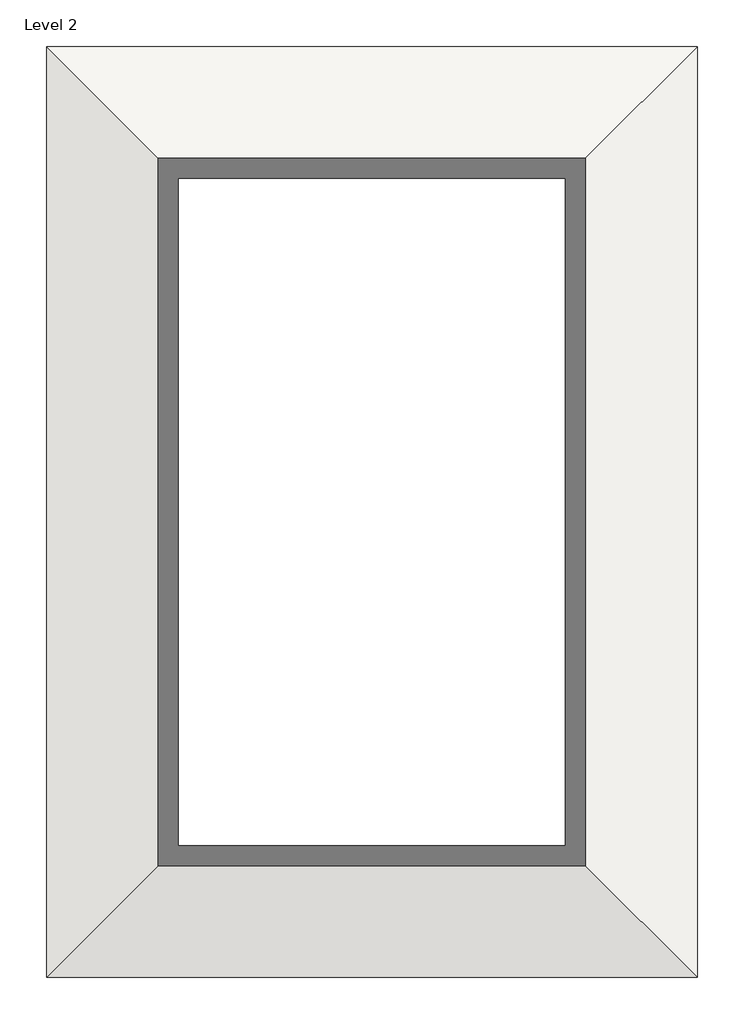
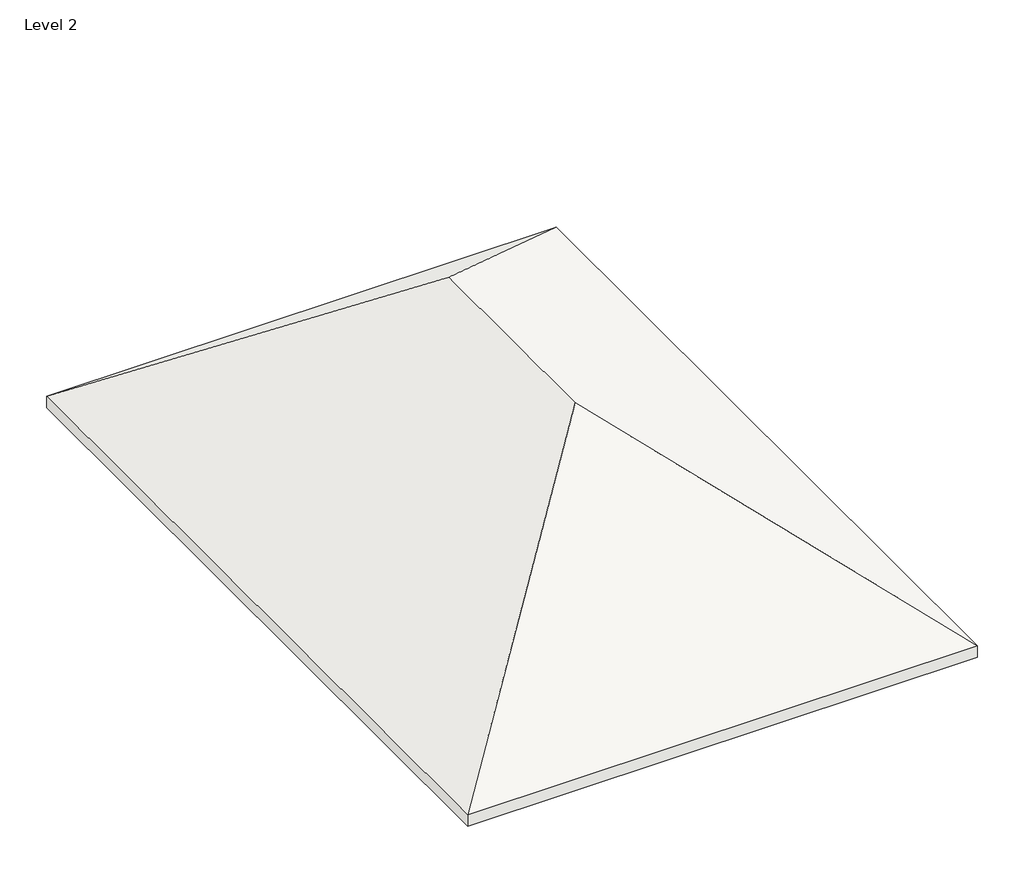
# One storey: 1 roof.
"""IFC4 building model written with IfcOpenShell, lengths in millimetres."""

from ifc_helpers import new_model, si_unit, origin, place, context, project, spatial, faceted_brep, element, save

model = new_model("IFC4")

# Units and contexts
model_context = context("Model", 3, world=origin())
ifc_project = project(units=[si_unit("LENGTHUNIT", "METRE", prefix="MILLI")], contexts=[model_context])

# Site, building, storey
site = spatial("IfcSite", under=ifc_project)
building = spatial("IfcBuilding", under=site)
storey = spatial("IfcBuildingStorey", under=building, Name="Level 2", Elevation=3048.0)

# Roof
placement = place(None, origin())
element("IfcRoof", 1, ObjectType="Generic - 12\"", at=placement, inside=storey, context=model_context, shape_type="Brep", body=[
    faceted_brep([(2670.5550833, 5769.3429147, 3048.0), (-1272.7949167, 1825.9929147, 6005.5125), (-5216.1449167, 5769.3429147, 3048.0), (-1272.7949167, -1564.9070853, 6005.5125), (-5216.1449167, -5508.2570853, 3048.0), (2670.5550833, -5508.2570853, 3048.0), (2670.5550833, 5769.3429147, 3238.5), (-5216.1449167, 5769.3429147, 3238.5), (-1272.7949167, 1825.9929147, 6196.0125), (-5216.1449167, -5508.2570853, 3238.5), (-1272.7949167, -1564.9070853, 6196.0125), (2670.5550833, -5508.2570853, 3238.5)], [[[0, 1, 2]], [[2, 1, 3, 4]], [[4, 3, 5]], [[1, 0, 5, 3]], [[6, 7, 8]], [[7, 9, 10, 8]], [[9, 11, 10]], [[6, 8, 10, 11]], [[2, 7, 6, 0]], [[4, 9, 7, 2]], [[5, 11, 9, 4]], [[0, 6, 11, 5]]]),
])

save(model, "model.ifc")

# Revit data of these elements
# Type "Generic - 12\""
#   Assembly Code = "B1020"
#   Layers, outside or top first: 0' - 6" no material (function 1)
# Element 1 (IfcRoof, "Generic - 12\"")
#   built-in parameter 1001705 = 20.3281 (stored number, unit not read)
#   built-in parameter 1001710 = 33615
#   Phase Created = New Construction
#   Materials on its faces: "Default Roof", "Blanket"
# Materials
#   "Default Roof": colour RGB 88 101 114, transparency 0, Cost = 0
#   "Blanket": class "System", colour RGB 59 0 1, transparency 0, Cost = 0
